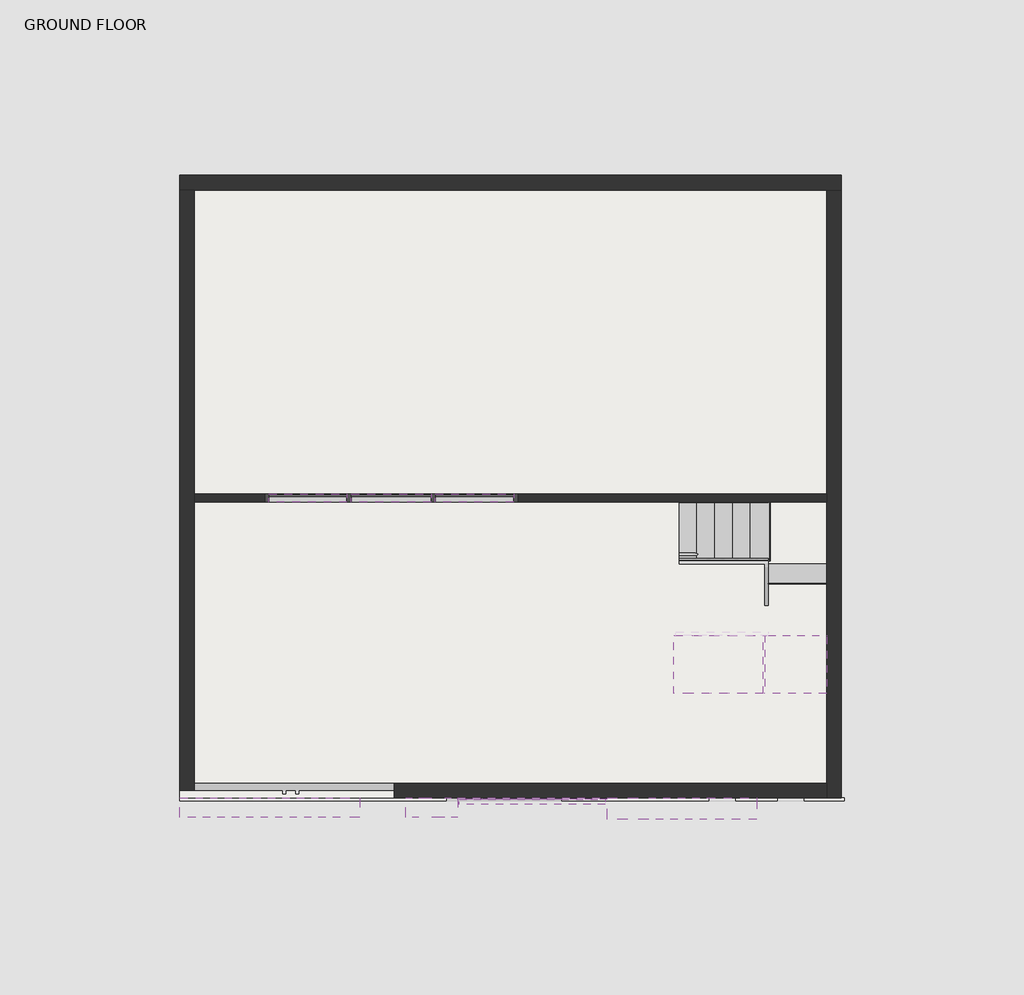
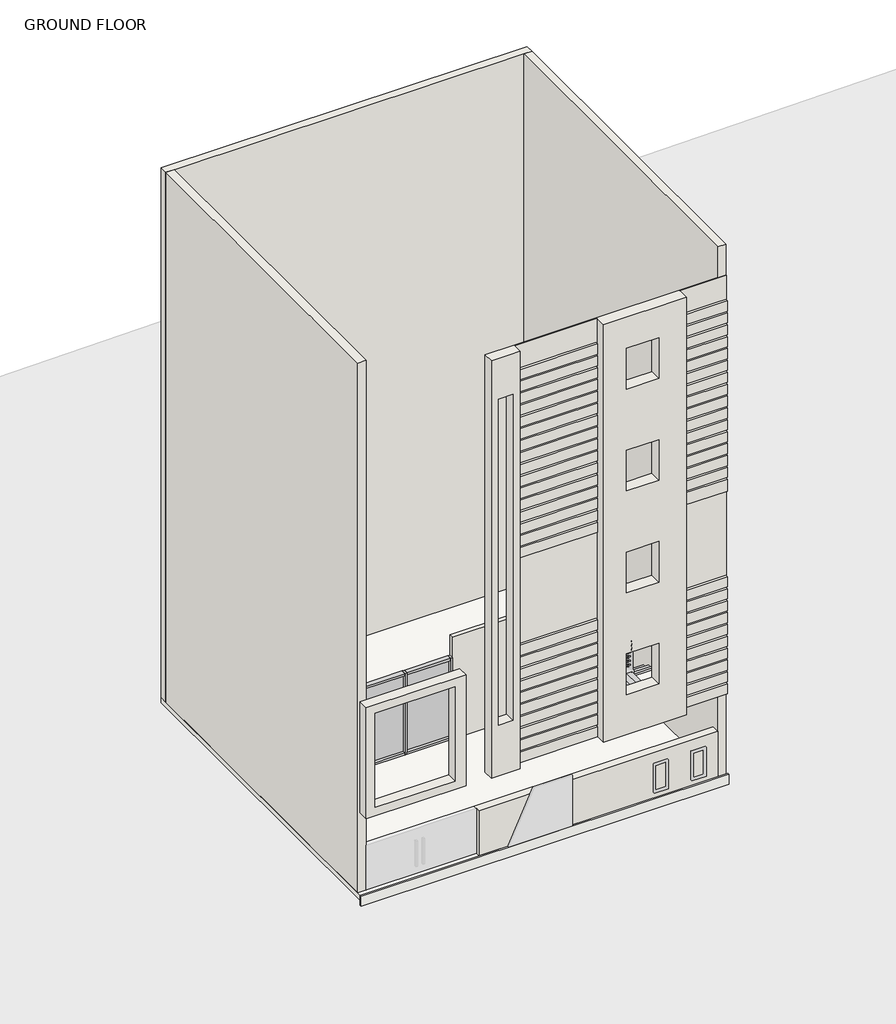
# One storey, part 1 of 3: 11 walls, 10 members, 4 slabs, 3 plates, 3 stair flights.
"""IFC4 building model written with IfcOpenShell, lengths in millimetres."""

from ifc_helpers import new_model, si_unit, frame, origin, place, context, project, spatial, polyline, outline, extrude, faceted_brep, transform, mapped, element, save
from components import member_86232e3a, member_30a5d983, member_f0fea5a5, member_ee409385, system_panel_glazed_6119edd6, system_panel_glazed_4edfead3, floors_2_floors_2_9b529a88, non_monolithic_landing_70e0e3a4, stair_flight_7b3f2189, stair_flight_6dcdbca7, stair_flight_b9a180af, walls_1_walls_1_8f4806b2, walls_2_walls_2_726db825, walls_3_walls_3_01008c03, walls_5_walls_5_43feafce, walls_6_walls_6_f5cc7341

model = new_model("IFC4")

# Units and contexts
model_context = context("Model", 3, world=origin())
ifc_project = project(units=[si_unit("LENGTHUNIT", "METRE", prefix="MILLI")], contexts=[model_context])

# Site, building, storey
site = spatial("IfcSite", under=ifc_project)
building = spatial("IfcBuilding", under=site)
storey = spatial("IfcBuildingStorey", under=building, Name="GROUND FLOOR", Elevation=304.8)

# Members
placement = place(None, origin())
member_shape = member_86232e3a(model_context)
element("IfcMember", 1, ObjectType="Rectangular Mullion : 2.5\" x 5\" rectangular", at=placement, inside=storey, context=model_context, shape_type="MappedRepresentation", body=[
    mapped(member_shape, transform((-1292.4569651, 5150.5055142, 2743.2), x_axis=(0.0, 0.0, 1.0), y_axis=(0.0, -1.0, 0.0), z_axis=(1.0, 0.0, 0.0))),
])
element("IfcMember", 2, ObjectType="Rectangular Mullion : 2.5\" x 5\" rectangular", at=placement, inside=storey, context=model_context, shape_type="MappedRepresentation", body=[
    mapped(member_shape, transform((-3902.306965, 5150.5055142, 2743.2), x_axis=(0.0, 0.0, 1.0), y_axis=(0.0, -1.0, 0.0), z_axis=(1.0, 0.0, 0.0))),
])
member_2_shape = member_30a5d983(model_context)
element("IfcMember", 3, ObjectType="Rectangular Mullion : 2.5\" x 5\" rectangular", at=placement, inside=storey, context=model_context, shape_type="MappedRepresentation", body=[
    mapped(member_2_shape, transform((-2581.5069652, 5150.5055142, 2743.2), x_axis=(0.0, 0.0, 1.0), y_axis=(0.0, -1.0, 0.0), z_axis=(1.0, 0.0, 0.0))),
])
element("IfcMember", 4, ObjectType="Rectangular Mullion : 2.5\" x 5\" rectangular", at=placement, inside=storey, context=model_context, shape_type="MappedRepresentation", body=[
    mapped(member_shape, transform((-5127.8569651, 5150.5055142, 304.8), x_axis=(0.0, 0.0, -1.0), y_axis=(0.0, -1.0, 0.0), z_axis=(-1.0, 0.0, 0.0))),
])
element("IfcMember", 5, ObjectType="Rectangular Mullion : 2.5\" x 5\" rectangular", at=placement, inside=storey, context=model_context, shape_type="MappedRepresentation", body=[
    mapped(member_shape, transform((-2518.0069652, 5150.5055142, 304.8), x_axis=(0.0, 0.0, -1.0), y_axis=(0.0, -1.0, 0.0), z_axis=(-1.0, 0.0, 0.0))),
])
element("IfcMember", 6, ObjectType="Rectangular Mullion : 2.5\" x 5\" rectangular", at=placement, inside=storey, context=model_context, shape_type="MappedRepresentation", body=[
    mapped(member_2_shape, transform((-3838.806965, 5150.5055142, 304.8), x_axis=(0.0, 0.0, -1.0), y_axis=(0.0, -1.0, 0.0), z_axis=(-1.0, 0.0, 0.0))),
])
member_3_shape = member_f0fea5a5(model_context)
element("IfcMember", 7, ObjectType="Rectangular Mullion : 2.5\" x 5\" rectangular", at=placement, inside=storey, context=model_context, shape_type="MappedRepresentation", body=[
    mapped(member_3_shape, transform((-3870.556965, 5150.5055142, 304.8), x_axis=(1.0, 0.0, 0.0), y_axis=(0.0, -1.0, 0.0), z_axis=(0.0, 0.0, -1.0))),
])
element("IfcMember", 8, ObjectType="Rectangular Mullion : 2.5\" x 5\" rectangular", at=placement, inside=storey, context=model_context, shape_type="MappedRepresentation", body=[
    mapped(member_3_shape, transform((-2549.7569652, 5150.5055142, 304.8), x_axis=(1.0, 0.0, 0.0), y_axis=(0.0, -1.0, 0.0), z_axis=(0.0, 0.0, -1.0))),
])
member_4_shape = member_ee409385(model_context)
element("IfcMember", 9, ObjectType="Rectangular Mullion : 2.5\" x 5\" rectangular", at=placement, inside=storey, context=model_context, shape_type="MappedRepresentation", body=[
    mapped(member_4_shape, transform((-1228.9569651, 5150.5055142, 304.8), x_axis=(1.0, 0.0, 0.0), y_axis=(0.0, -1.0, 0.0), z_axis=(0.0, 0.0, -1.0))),
])
element("IfcMember", 10, ObjectType="Rectangular Mullion : 2.5\" x 5\" rectangular", at=placement, inside=storey, context=model_context, shape_type="MappedRepresentation", body=[
    mapped(member_4_shape, transform((-5191.3569651, 5150.5055142, 2743.2), x_axis=(-1.0, 0.0, 0.0), y_axis=(0.0, -1.0, 0.0), z_axis=(0.0, 0.0, 1.0))),
])

# Plates
system_panel_glazed_shape = system_panel_glazed_6119edd6(model_context)
element("IfcPlate", 11, ObjectType="System Panel : Glazed", at=placement, inside=storey, context=model_context, shape_type="MappedRepresentation", body=[
    mapped(system_panel_glazed_shape, transform((-4515.081965, 5150.5055142, 368.3), x_axis=(1.0, 0.0, 0.0), y_axis=(0.0, 1.0, 0.0), z_axis=(0.0, 0.0, 1.0))),
])
element("IfcPlate", 12, ObjectType="System Panel : Glazed", at=placement, inside=storey, context=model_context, shape_type="MappedRepresentation", body=[
    mapped(system_panel_glazed_shape, transform((-1905.2319651, 5150.5055142, 368.3), x_axis=(1.0, 0.0, 0.0), y_axis=(0.0, 1.0, 0.0), z_axis=(0.0, 0.0, 1.0))),
])
system_panel_glazed_2_shape = system_panel_glazed_4edfead3(model_context)
element("IfcPlate", 13, ObjectType="System Panel : Glazed", at=placement, inside=storey, context=model_context, shape_type="MappedRepresentation", body=[
    mapped(system_panel_glazed_2_shape, transform((-3210.1569651, 5150.5055142, 368.3), x_axis=(1.0, 0.0, 0.0), y_axis=(0.0, 1.0, 0.0), z_axis=(0.0, 0.0, 1.0))),
])

# Slabs
floors_2_floors_2_shape = floors_2_floors_2_9b529a88(model_context)
element("IfcSlab", 14, ObjectType="Floors 2 : Floors 2", at=placement, inside=storey, context=model_context, shape_type="MappedRepresentation", body=[
    mapped(floors_2_floors_2_shape, transform((0.0, 0.0, 0.0), x_axis=(1.0, 0.0, 0.0), y_axis=(0.0, 1.0, 0.0), z_axis=(0.0, 0.0, 1.0))),
])
element("IfcSlab", 15, ObjectType="Generic - 12\"", at=placement, inside=storey, context=model_context, shape_type="SweptSolid", body=[
    extrude(outline(polyline([(3838.3430349, 10205.1055142), (3838.3430349, 451.5055142), (-6524.8569651, 451.5055142), (-6524.8569651, 10205.1055142), (3838.3430349, 10205.1055142)])), frame((0.0, 0.0, 152.4), z_axis=(0.0, 0.0, 1.0), x_axis=(1.0, 0.0, 0.0)), (0.0, 0.0, 1.0), 152.4),
])
element("IfcSlab", 16, ObjectType="Generic - 12\"", at=placement, inside=storey, context=model_context, shape_type="SweptSolid", body=[
    extrude(outline(polyline([(3838.3430349, 10205.1055142), (3838.3430349, 451.5055142), (-6524.8569651, 451.5055142), (-6524.8569651, 10205.1055142), (3838.3430349, 10205.1055142)])), frame((0.0, 0.0, 152.4), z_axis=(0.0, 0.0, 1.0), x_axis=(1.0, 0.0, 0.0)), (0.0, 0.0, 1.0), 152.4),
])
non_monolithic_landing_shape = non_monolithic_landing_70e0e3a4(model_context)
element("IfcSlab", 17, ObjectType="Non-Monolithic Landing", at=placement, inside=storey, context=model_context, shape_type="MappedRepresentation", body=[
    mapped(non_monolithic_landing_shape, transform((0.0, 0.0, 0.0), x_axis=(1.0, 0.0, 0.0), y_axis=(0.0, 1.0, 0.0), z_axis=(0.0, 0.0, 1.0))),
])

# Stair flights
stair_flight_shape = stair_flight_7b3f2189(model_context)
element("IfcStairFlight", 18, ObjectType="2\" Tread 1\" Nosing 1/4\" Riser", at=placement, inside=storey, context=model_context, shape_type="MappedRepresentation", body=[
    mapped(stair_flight_shape, transform((0.0, 0.0, 0.0), x_axis=(1.0, 0.0, 0.0), y_axis=(0.0, 1.0, 0.0), z_axis=(0.0, 0.0, 1.0))),
])
stair_flight_2_shape = stair_flight_6dcdbca7(model_context)
element("IfcStairFlight", 19, ObjectType="2\" Tread 1\" Nosing 1/4\" Riser", at=placement, inside=storey, context=model_context, shape_type="MappedRepresentation", body=[
    mapped(stair_flight_2_shape, transform((0.0, 0.0, 0.0), x_axis=(1.0, 0.0, 0.0), y_axis=(0.0, 1.0, 0.0), z_axis=(0.0, 0.0, 1.0))),
])
stair_flight_3_shape = stair_flight_b9a180af(model_context)
element("IfcStairFlight", 20, ObjectType="2\" Tread 1\" Nosing 1/4\" Riser", at=placement, inside=storey, context=model_context, shape_type="MappedRepresentation", body=[
    mapped(stair_flight_3_shape, transform((0.0, 0.0, 0.0), x_axis=(1.0, 0.0, 0.0), y_axis=(0.0, 1.0, 0.0), z_axis=(0.0, 0.0, 1.0))),
])

# Walls
element("IfcWall", 21, ObjectType="5\"", at=placement, inside=storey, context=model_context, shape_type="SweptSolid", body=[
    extrude(outline(polyline([(-5191.3569651, 5087.0055142), (-6296.2569651, 5087.0055142), (-6296.2569651, 5214.0055142), (-5191.3569651, 5214.0055142), (-5191.3569651, 5087.0055142)])), frame((0.0, 0.0, 304.8), z_axis=(0.0, 0.0, 1.0), x_axis=(1.0, 0.0, 0.0)), (0.0, 0.0, 1.0), 3048.0),
])
element("IfcWall", 22, ObjectType="5\"", at=placement, inside=storey, context=model_context, shape_type="SweptSolid", body=[
    extrude(outline(polyline([(3609.7430349, 5087.0055142), (-1228.9569651, 5087.0055142), (-1228.9569651, 5214.0055142), (3609.7430349, 5214.0055142), (3609.7430349, 5087.0055142)])), frame((0.0, 0.0, 304.8), z_axis=(0.0, 0.0, 1.0), x_axis=(1.0, 0.0, 0.0)), (0.0, 0.0, 1.0), 3048.0),
])
element("IfcWall", 23, ObjectType="9\"", at=placement, inside=storey, context=model_context, shape_type="Brep", body=[
    faceted_brep([(-6524.8569651, 9976.5055142, 304.8), (-6296.2569651, 9976.5055142, 304.8), (3609.7430349, 9976.5055142, 304.8), (3838.3430349, 9976.5055142, 304.8), (3838.3430349, 9976.5055142, 16154.4), (3609.7430349, 9976.5055142, 16154.4), (-6296.2569651, 9976.5055142, 16154.4), (-6524.8569651, 9976.5055142, 16154.4), (-6524.8569651, 10205.1055142, 304.8), (-6524.8569651, 10205.1055142, 16154.4), (3838.3430349, 10205.1055142, 16154.4), (3838.3430349, 10205.1055142, 304.8)], [[[0, 1, 2, 3, 4, 5, 6, 7]], [[8, 9, 10, 11]], [[3, 2, 1, 0, 8, 11]], [[7, 6, 5, 4, 10, 9]], [[4, 3, 11, 10]], [[0, 7, 9, 8]]]),
])
element("IfcWall", 24, ObjectType="9\"", at=placement, inside=storey, context=model_context, shape_type="Brep", body=[
    faceted_brep([(3609.7430349, 9976.5055142, 304.8), (3609.7430349, 5214.0055142, 304.8), (3609.7430349, 5087.0055142, 304.8), (3609.7430349, 680.1055142, 304.8), (3609.7430349, 451.5055142, 304.8), (3609.7430349, 451.5055142, 1653.0575529), (3609.7430349, 451.5055142, 3048.0), (3609.7430349, 451.5055142, 15240.0), (3609.7430349, 451.5055142, 16154.4), (3609.7430349, 680.1055142, 16154.4), (3609.7430349, 9976.5055142, 16154.4), (3838.3430349, 9976.5055142, 304.8), (3838.3430349, 9976.5055142, 16154.4), (3838.3430349, 451.5055142, 16154.4), (3838.3430349, 451.5055142, 304.8)], [[[0, 1, 2, 3, 4, 5, 6, 7, 8, 9, 10]], [[11, 12, 13, 14]], [[4, 3, 2, 1, 0, 11, 14]], [[10, 9, 8, 13, 12]], [[0, 10, 12, 11]], [[4, 14, 13, 8, 7, 6, 5]]]),
])
element("IfcWall", 25, ObjectType="9\"", at=placement, inside=storey, context=model_context, shape_type="Brep", body=[
    faceted_brep([(-6296.2569651, 565.8055142, 304.8), (-6296.2569651, 5087.0055142, 304.8), (-6296.2569651, 5214.0055142, 304.8), (-6296.2569651, 9976.5055142, 304.8), (-6296.2569651, 9976.5055142, 16154.4), (-6296.2569651, 565.8055142, 16154.4), (-6524.8569651, 565.8055142, 304.8), (-6524.8569651, 565.8055142, 16154.4), (-6524.8569651, 9976.5055142, 16154.4), (-6524.8569651, 9976.5055142, 304.8)], [[[0, 1, 2, 3, 4, 5]], [[6, 7, 8, 9]], [[3, 2, 1, 0, 6, 9]], [[5, 4, 8, 7]], [[0, 5, 7, 6]], [[4, 3, 9, 8]]]),
])
element("IfcWall", 26, ObjectType="9\"", at=placement, inside=storey, context=model_context, shape_type="SweptSolid", body=[
    extrude(outline(polyline([(3609.7430349, 451.5055142), (-3159.3569651, 451.5055142), (-3159.3569651, 680.1055142), (3609.7430349, 680.1055142), (3609.7430349, 451.5055142)])), frame((0.0, 0.0, 304.8), z_axis=(0.0, 0.0, 1.0), x_axis=(1.0, 0.0, 0.0)), (0.0, 0.0, 1.0), 1348.2575529),
])
walls_1_walls_1_shape = walls_1_walls_1_8f4806b2(model_context)
element("IfcWall", 27, ObjectType="Walls 1 : Walls 1", at=placement, inside=storey, context=model_context, shape_type="MappedRepresentation", body=[
    mapped(walls_1_walls_1_shape, transform((0.0, 0.0, 0.0), x_axis=(1.0, 0.0, 0.0), y_axis=(0.0, 1.0, 0.0), z_axis=(0.0, 0.0, 1.0))),
])
walls_2_walls_2_shape = walls_2_walls_2_726db825(model_context)
element("IfcWall", 28, ObjectType="Walls 2 : Walls 2", at=placement, inside=storey, context=model_context, shape_type="MappedRepresentation", body=[
    mapped(walls_2_walls_2_shape, transform((0.0, 0.0, 0.0), x_axis=(1.0, 0.0, 0.0), y_axis=(0.0, 1.0, 0.0), z_axis=(0.0, 0.0, 1.0))),
])
walls_3_walls_3_shape = walls_3_walls_3_01008c03(model_context)
element("IfcWall", 29, ObjectType="Walls 3 : Walls 3", at=placement, inside=storey, context=model_context, shape_type="MappedRepresentation", body=[
    mapped(walls_3_walls_3_shape, transform((0.0, 0.0, 0.0), x_axis=(1.0, 0.0, 0.0), y_axis=(0.0, 1.0, 0.0), z_axis=(0.0, 0.0, 1.0))),
])
walls_5_walls_5_shape = walls_5_walls_5_43feafce(model_context)
element("IfcWall", 30, ObjectType="Walls 5 : Walls 5", at=placement, inside=storey, context=model_context, shape_type="MappedRepresentation", body=[
    mapped(walls_5_walls_5_shape, transform((0.0, 0.0, 0.0), x_axis=(1.0, 0.0, 0.0), y_axis=(0.0, 1.0, 0.0), z_axis=(0.0, 0.0, 1.0))),
])
walls_6_walls_6_shape = walls_6_walls_6_f5cc7341(model_context)
element("IfcWall", 31, ObjectType="Walls 6 : Walls 6", at=placement, inside=storey, context=model_context, shape_type="MappedRepresentation", body=[
    mapped(walls_6_walls_6_shape, transform((0.0, 0.0, 0.0), x_axis=(1.0, 0.0, 0.0), y_axis=(0.0, 1.0, 0.0), z_axis=(0.0, 0.0, 1.0))),
])

save(model, "model.ifc")

# Revit data of these elements
# Type "Rectangular Mullion : 2.5\" x 5\" rectangular"
#   built-in parameter 1007304 = 0.416667 (stored number, unit not read)
#   built-in parameter 1007301 = 0.104167 (stored number, unit not read)
#   built-in parameter 1007300 = 0.104167 (stored number, unit not read)
# Type "System Panel : Glazed"
#   Construction Type Id = "GSP4R"
#   Analytic Construction = "1/8 in Pilkington single glazing"
#   Visual Light Transmittance = 0.9
#   Solar Heat Gain Coefficient = 0.86
#   Heat Transfer Coefficient (U) = 1.18115 BTU/(h·ft²·°F)
#   Define Thermal Properties by = 1
# Type "Generic - 12\""
#   Assembly Code = "B1010"
#   Function = 0
#   Layers, outside or top first: 0' - 6" no material (function 1)
# Type "5\""
#   Assembly Code = "B2010"
#   Layers, outside or top first: 0' - 5" "Concrete Masonry Units" (function 1)
# Type "9\""
#   Assembly Code = "B2010"
#   Layers, outside or top first: 0' - 9" no material (function 1)
# Elements 1, 2, 3, 4, 5, 6, 7, 8, 9, 10 (IfcMember, "Rectangular Mullion : 2.5\" x 5\" rectangular")
#   Phase Created = New Construction
#   Materials on its faces: "Aluminum"
# Elements 11, 12, 13 (IfcPlate, "System Panel : Glazed")
#   Phase Created = New Construction
#   Materials on its faces: "Glass"
# Element 14 (IfcSlab, "Floors 2 : Floors 2")
#   Phase Created = New Construction
#   Materials on its faces: "1 wall brown", "Default Floor"
# Element 15 (IfcSlab, "Generic - 12\"")
#   Height Offset From Level = 0' - 0"
#   Phase Created = New Construction
#   Materials on its faces: "Default Floor"
# Element 16 (IfcSlab, "Generic - 12\"")
#   Height Offset From Level = 0' - 0"
#   Phase Created = New Construction
#   Materials on its faces: "Default Floor", "1 wall brown"
# Element 17 (IfcSlab, "Non-Monolithic Landing")
#   Phase Created = New Construction
# Elements 18, 19, 20 (IfcStairFlight, "2\" Tread 1\" Nosing 1/4\" Riser")
#   Phase Created = New Construction
# Elements 21, 22 (IfcWall, "5\"")
#   Top Offset = 0' - 0"
#   Base Offset = 0' - 0"
#   Unconnected Height = 10' - 0"
#   wall height = 10' - 0"
#   Phase Created = New Construction
#   Base Constraint = GROUND FLOOR
#   Materials on its faces: "Concrete Masonry Units", "1 wall white"
# Element 23 (IfcWall, "9\"")
#   Top Offset = 0' - 0"
#   Base Offset = 0' - 0"
#   Unconnected Height = 52' - 0"
#   wall height = 52' - 0"
#   Phase Created = New Construction
#   Base Constraint = GROUND FLOOR
#   Materials on its faces: "1 wall white", "Default Wall"
# Elements 24, 25 (IfcWall, "9\"")
#   Top Offset = 0' - 0"
#   Base Offset = 0' - 0"
#   Unconnected Height = 52' - 0"
#   wall height = 52' - 0"
#   Phase Created = New Construction
#   Base Constraint = GROUND FLOOR
#   Materials on its faces: "1 wall white", "Default Wall", "1 wall brown"
# Element 26 (IfcWall, "9\"")
#   Top Offset = 0' - 0"
#   Base Offset = 0' - 0"
#   Unconnected Height = 4' - 5.08101"
#   wall height = 4' - 5.08101"
#   Phase Created = New Construction
#   Base Constraint = GROUND FLOOR
#   Materials on its faces: "Default Wall", "1 wall white"
# Element 27 (IfcWall, "Walls 1 : Walls 1")
#   Phase Created = New Construction
#   Materials on its faces: "1 wall brown", "Default Wall"
# Element 28 (IfcWall, "Walls 2 : Walls 2")
#   Phase Created = New Construction
#   Materials on its faces: "1 wall white", "Default Wall"
# Element 29 (IfcWall, "Walls 3 : Walls 3")
#   Phase Created = New Construction
#   Materials on its faces: "1 wall white", "Default Wall"
# Element 30 (IfcWall, "Walls 5 : Walls 5")
#   Phase Created = New Construction
#   Materials on its faces: "Default Wall", "1 wall white"
# Element 31 (IfcWall, "Walls 6 : Walls 6")
#   Phase Created = New Construction
#   Materials on its faces: "Default Wall", "1 wood"
# Materials
#   "Concrete Masonry Units": class "Masonry", colour RGB 227 227 227, transparency 0, Description = "Concrete masonry units", Cost = 0
#   "Aluminum": class "Metal", colour RGB 247 247 247, transparency 0, Description = "Aluminum 6061", Cost = 0
#   "Glass": class "Glass", colour RGB 0 128 192, transparency 0.75, Description = "Soda Lime Glass", Cost = 0
#   "1 wall brown": class "Generic", colour RGB 61 46 37, transparency 0, Cost = 0
#   "Default Floor": colour RGB 128 128 128, transparency 0, Cost = 0
#   "1 wall white": class "Generic", colour RGB 244 245 241, transparency 0, Cost = 0
#   "Default Wall": colour RGB 128 128 128, transparency 0, Cost = 0
#   "1 wood": class "Generic", colour RGB 120 120 120, transparency 0, Cost = 0
